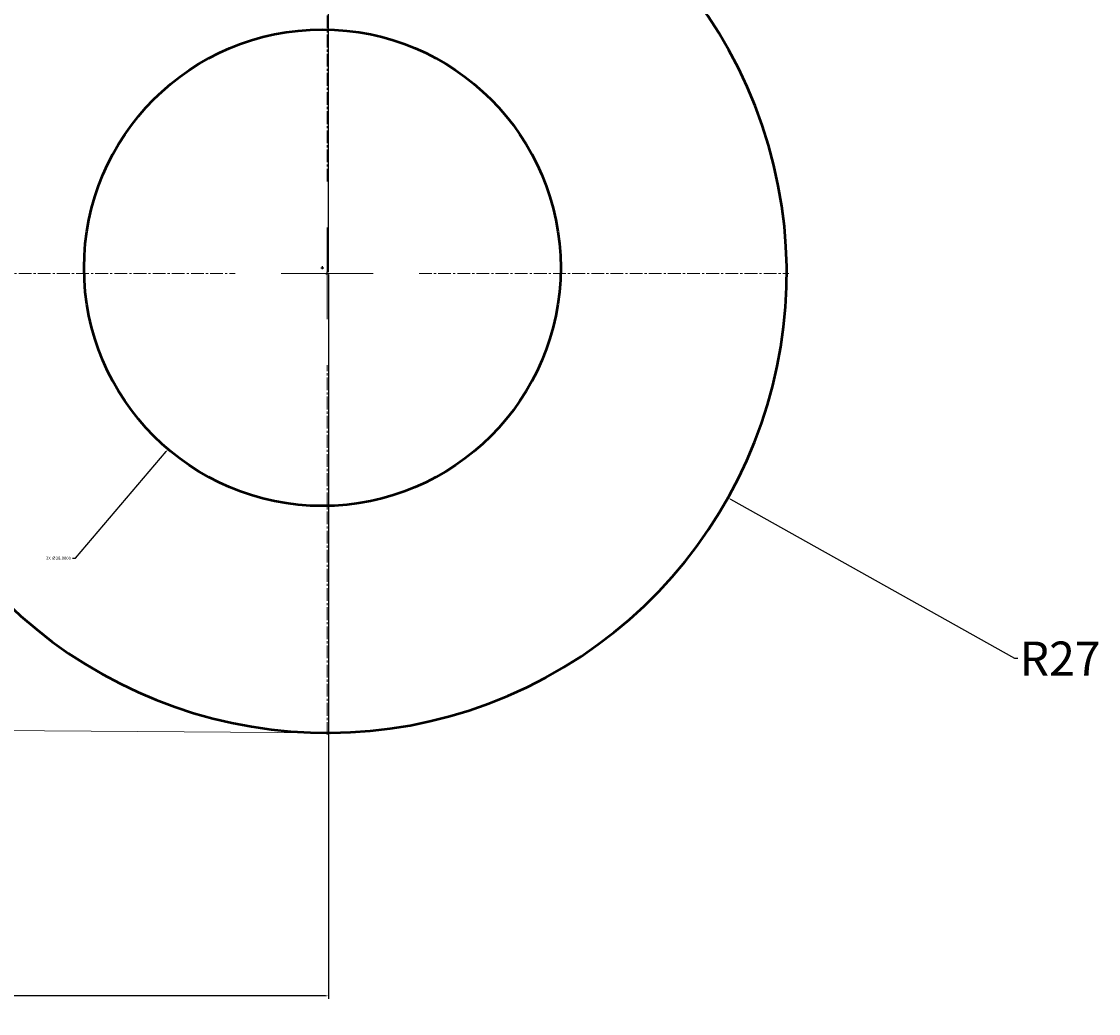
# Model space of a CAD drawing. Units: millimetres. Extents: x -60 to 113, y -37 to 126.
# Tile 16 of 17: x 49 to 113, y -37 to 21. Entities that reach past the tile are written whole.
import ezdxf

# ---------------------------------------------------------------- set-up
doc = ezdxf.new("R2010")
doc.units = ezdxf.units.MM
doc.header["$MEASUREMENT"] = 0
doc.linetypes.add('CENTER2', pattern=[1.125, 0.75, -0.125, 0.125, -0.125])
for name, color, linetype, lineweight in [('M-CNTR', 4, 'CENTER2', 18), ('M-CONS', 8, 'Continuous', 13), ('M-DIMS', 2, 'Continuous', 25), ('M-OUTL', 7, 'Continuous', 50)]:
    doc.layers.add(name, color=color, linetype=linetype, lineweight=lineweight)
doc.styles.get("Standard").update_dxf_attribs({"font": 'arial.ttf'})
doc.dimstyles.get("Standard").update_dxf_attribs({"dimtxt": 0.18, "dimasz": 0.18, "dimexe": 0.18, "dimexo": 0.0625, "dimgap": 0.09, "dimtad": 0, "dimtih": 1, "dimtoh": 1, "dimdec": 4, "dimzin": 0, "dimdsep": 46, "dimtxsty": 'Standard', "dimcen": 0.09, "dimadec": 0, "dimazin": 0, "dimtfac": 1, "dimtdec": 4, "dimtofl": 0, "dimtmove": 0, "dimatfit": 3, "dimfxl": 1, "dimtolj": 1, "dimtzin": 0, "dimarcsym": 0})

# ---------------------------------------------------------------- blocks, each defined once
blk = doc.blocks.new('*U3')
at = {"layer": 'M-CNTR', "color": 0, "transparency": 16777216}
for p, q in [((0, 5.4), (0, 27.12)), ((-27.12, 0), (-5.4, 0)), ((5.4, 0), (27.12, 0)), ((0, -27.12), (0, -5.4))]:
    blk.add_line(p, q, dxfattribs=at)
at = {"layer": 'M-CNTR', "color": 0, "linetype": 'Continuous', "transparency": 16777216}
for p, q in [((0, -2.7), (0, 2.7)), ((-2.7, 0), (2.7, 0))]:
    blk.add_line(p, q, dxfattribs=at)
blk = doc.blocks.new('*D5')
at = {"layer": 'Defpoints', "color": 0, "transparency": 16777216}
for p in [(67.265, 6.442), (90.82, -6.755)]:
    blk.add_point(p, dxfattribs=at)
at = {"layer": 'M-DIMS', "color": 0, "lineweight": -2, "transparency": 16777216}
for p, q in [((67.175, 6.442), (67.355, 6.442)), ((67.265, 6.352), (67.265, 6.532)), ((107.668, -16.194), (90.977, -6.843)), ((107.848, -16.194), (107.668, -16.194))]:
    blk.add_line(p, q, dxfattribs=at)
at = {"layer": 'M-DIMS', "color": 0, "transparency": 16777216}
blk.add_solid([(90.992, -6.816), (90.963, -6.869), (90.82, -6.755)], dxfattribs=at)
at = {"layer": 'M-DIMS', "color": 0, "transparency": 16777216, "insert": (110.328, -16.194), "char_height": 0.18, "attachment_point": 5}
blk.add_mtext('\\A1;{\\H11.11111x;R27}', dxfattribs=at)
blk = doc.blocks.new('*D14')
at = {"layer": 'Defpoints', "color": 0, "transparency": 16777216}
for p in [(7.267, 6.903), (67.355, 6.442), (67.355, -36.011)]:
    blk.add_point(p, dxfattribs=at)
at = {"layer": 'M-DIMS', "color": 0, "lineweight": -2, "transparency": 16777216}
for p, q in [((7.267, 6.84), (7.267, -36.191)), ((67.355, 6.379), (67.355, -36.191)), ((7.447, -36.011), (35.786, -36.011)), ((67.175, -36.011), (38.835, -36.011))]:
    blk.add_line(p, q, dxfattribs=at)
at = {"layer": 'M-DIMS', "color": 0, "transparency": 16777216}
for points in [[(7.447, -35.981), (7.447, -36.041), (7.267, -36.011)], [(67.175, -35.981), (67.175, -36.041), (67.355, -36.011)]]:
    blk.add_solid(points, dxfattribs=at)
at = {"layer": 'M-DIMS', "color": 0, "transparency": 16777216, "insert": (37.311, -36.011), "char_height": 0.18, "attachment_point": 5}
blk.add_mtext('\\A1;{\\H11.11111x;60}', dxfattribs=at)
blk = doc.blocks.new('*D17')
at = {"layer": 'Defpoints', "color": 0, "transparency": 16777216}
for p in [(67.355, 124.823), (10.532, 88.533), (67.355, 6.442)]:
    blk.add_point(p, dxfattribs=at)
at = {"layer": 'M-DIMS', "color": 0, "lineweight": -2, "transparency": 16777216}
for p, q in [((10.532, 88.595), (10.532, 125.003)), ((10.712, 124.823), (37.422, 124.823)), ((67.175, 124.823), (40.465, 124.823)), ((67.355, 6.504), (67.355, 125.003))]:
    blk.add_line(p, q, dxfattribs=at)
at = {"layer": 'M-DIMS', "color": 0, "transparency": 16777216}
for points in [[(10.712, 124.853), (10.712, 124.793), (10.532, 124.823)], [(67.175, 124.853), (67.175, 124.793), (67.355, 124.823)]]:
    blk.add_solid(points, dxfattribs=at)
at = {"layer": 'M-DIMS', "color": 0, "transparency": 16777216, "insert": (38.944, 124.823), "char_height": 0.18, "attachment_point": 5}
blk.add_mtext('\\A1;{\\H11.11111x;56}', dxfattribs=at)
blk = doc.blocks.new('HOLE-D28')
blk.add_circle((14, 14), 14)
blk = doc.blocks.new('*D21')
at = {"layer": 'Defpoints', "color": 0, "transparency": 16777216}
for p in [(76.053, 17.44), (57.919, -3.895)]:
    blk.add_point(p, dxfattribs=at)
at = {"layer": 'M-DIMS', "color": 0, "lineweight": -2, "transparency": 16777216}
for p, q in [((66.896, 6.773), (67.076, 6.773)), ((66.986, 6.683), (66.986, 6.863)), ((52.479, -10.295), (57.803, -4.032)), ((52.299, -10.295), (52.479, -10.295))]:
    blk.add_line(p, q, dxfattribs=at)
at = {"layer": 'M-DIMS', "color": 0, "transparency": 16777216}
blk.add_solid([(57.78, -4.013), (57.826, -4.052), (57.919, -3.895)], dxfattribs=at)
at = {"layer": 'M-DIMS', "color": 0, "transparency": 16777216, "insert": (51.48, -10.295), "char_height": 0.18, "attachment_point": 5}
blk.add_mtext('\\A1;3X ∅28.0000', dxfattribs=at)

msp = doc.modelspace()

# ---------------------------------------------------------------- linework, layer by layer
at = {"layer": 'M-CONS'}
msp.add_line((7.05918, -20.09651), (67.05741, -20.55741), dxfattribs=at)
at = {"layer": 'M-OUTL'}
msp.add_arc((67.26481, 6.44179), 27, 215.3846391, 96.5826838, dxfattribs=at)

# ---------------------------------------------------------------- block references
at = {"layer": 'M-CNTR'}
msp.add_blockref('*U3', (67.26481, 6.44179), dxfattribs=at)
at = {"layer": 'M-OUTL'}
msp.add_blockref('HOLE-D28', (52.98634, -7.22712), dxfattribs=at)

# ---------------------------------------------------------------- dimensions: what is measured, and where the dimension line sits
at = {"layer": 'M-DIMS'}
for base, p1, text, picture, middle in [((67.35481, 124.82251), (10.53227, 88.53289), '{\\H11.11111x;56}', '*D17', (38.94354, 124.82251)), ((67.35481, -36.0105), (7.26659, 6.9027), '{\\H11.11111x;60}', '*D14', (37.3107, -36.0105))]:
    dim = msp.add_linear_dim(base=base, p1=p1, p2=(67.35481, 6.44179), text=text, dimstyle='Standard', override={"dimclrd": 0, "dimclre": 0, "dimclrt": 0}, dxfattribs=at)
    dim.commit()
    dim.dimension.update_dxf_attribs({"geometry": picture, "text_midpoint": middle})
dim = msp.add_diameter_dim_2p(p1=(76.05255, 17.44011), p2=(57.91929, -3.89496), text='3X <>', dimstyle='Standard', override={"dimdec": 4, "dimlfac": 1, "dimrnd": 0, "dimzin": 0, "dimdsep": 46, "dimlunit": 2}, dxfattribs=at)
dim.commit()
dim.dimension.update_dxf_attribs({"geometry": '*D21', "text_midpoint": (51.47962, -10.29548), "dimtype": 163})
dim = msp.add_radius_dim(center=(67.26481, 6.44179), mpoint=(90.82015, -6.75465), text='{\\H11.11111x;R27}', dimstyle='Standard', override={"dimclrd": 0, "dimclre": 0, "dimclrt": 0}, dxfattribs=at)
dim.commit()
dim.dimension.update_dxf_attribs({"geometry": '*D5', "text_midpoint": (110.32798, -16.19361), "dimtype": 164})

doc.saveas('drawing.dxf')
